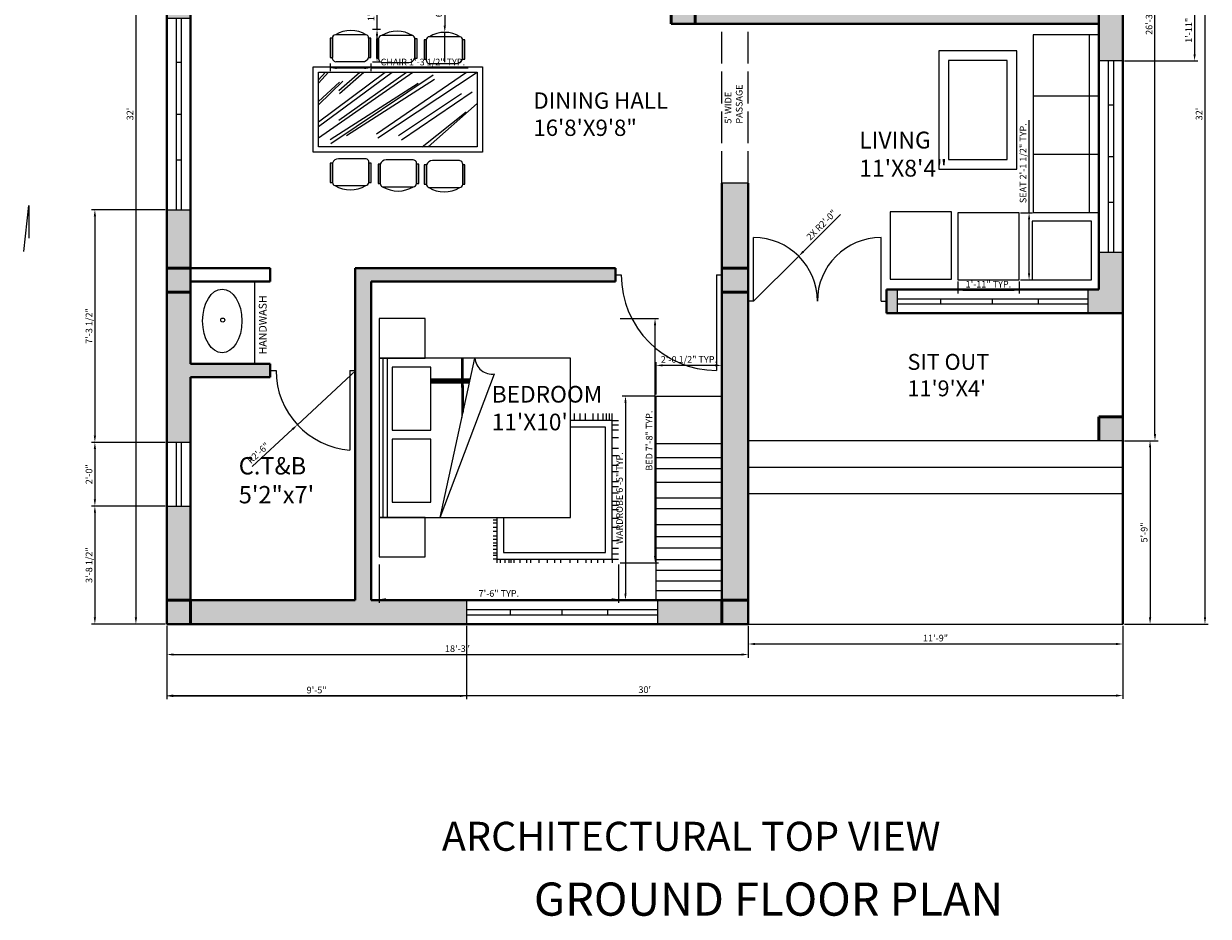
# Model space of a CAD drawing. Units: inches. Extents: x 599 to 1046, y 473 to 1020.
# Tile 1 of 2: x 599 to 1046, y 473 to 809. Entities that reach past the tile are written whole.
import ezdxf

# ---------------------------------------------------------------- set-up
doc = ezdxf.new("R2010")
doc.units = ezdxf.units.IN
doc.linetypes.add('ACAD_ISO02W100', pattern=[15, 12, -3])
for name, color, linetype, lineweight in [('A-ANNO-DIMS', 2, 'Continuous', 18), ('A-ANNO-MARK', 1, 'Continuous', 18), ('A-ANNO-TITL', 7, 'Continuous', 35), ('A-AREA-IDEN', 7, 'Continuous', 25), ('A-COLS', 7, 'Continuous', 50), ('A-COLS-PATT', 1, 'Continuous', 13), ('A-DOOR', 3, 'Continuous', 25), ('A-FLOR', 7, 'Continuous', 25), ('A-FLOR-CASE', 8, 'Continuous', 20), ('A-FLOR-FIXT', 9, 'Continuous', 18), ('A-FLOR-OVHD', 7, 'ACAD_ISO02W100', 18), ('A-FLOR-STRS', 7, 'Continuous', 25), ('A-FURN', 8, 'Continuous', 18), ('A-GLAZ', 4, 'Continuous', 18), ('A-WALL', 7, 'Continuous', 40), ('A-WALL-PATT', 252, 'Continuous', 13)]:
    doc.layers.add(name, color=color, linetype=linetype, lineweight=lineweight)
doc.styles.get("Standard").update_dxf_attribs({"font": 'arial.ttf'})
doc.dimstyles.new('ISO-25', dxfattribs={"dimtxt": 2.5, "dimasz": 2.5, "dimexe": 1.25, "dimexo": 0.625, "dimtad": 1, "dimdec": 0, "dimlunit": 3, "dimtxsty": 'Standard', "dimcen": 2.5, "dimadec": 0, "dimazin": 0, "dimtfac": 1, "dimtdec": 0, "dimtmove": 0, "dimatfit": 3, "dimfxl": 1, "dimarcsym": 0})

# ---------------------------------------------------------------- blocks, each defined once
blk = doc.blocks.new('*D2')
at = {"layer": 'A-ANNO-DIMS', "color": 0, "lineweight": -2, "transparency": 16777216}
for p, q in [((653.31, 582.63), (653.31, 570.57)), ((872.31, 582.63), (872.31, 570.57)), ((655.81, 571.82), (869.81, 571.82))]:
    blk.add_line(p, q, dxfattribs=at)
at = {"layer": 'A-ANNO-DIMS', "color": 0, "transparency": 16777216}
for points in [[(655.81, 572.23), (655.81, 571.4), (653.31, 571.82)], [(869.81, 572.23), (869.81, 571.4), (872.31, 571.82)]]:
    blk.add_solid(points, dxfattribs=at)
at = {"layer": 'Defpoints', "color": 0, "transparency": 16777216}
for p in [(653.31, 583.26), (872.31, 583.26), (872.31, 571.82)]:
    blk.add_point(p, dxfattribs=at)
at = {"layer": 'A-ANNO-DIMS', "color": 0, "transparency": 16777216, "insert": (762.81, 573.72), "char_height": 2.5, "attachment_point": 5}
blk.add_mtext('18\'-3"', dxfattribs=at)
blk = doc.blocks.new('*D3')
at = {"layer": 'A-ANNO-DIMS', "color": 0, "lineweight": -2, "transparency": 16777216}
for p, q in [((872.31, 582.63), (872.31, 574.53)), ((1013.31, 582.63), (1013.31, 574.53)), ((874.81, 575.78), (1010.81, 575.78))]:
    blk.add_line(p, q, dxfattribs=at)
at = {"layer": 'A-ANNO-DIMS', "color": 0, "transparency": 16777216}
for points in [[(874.81, 576.19), (874.81, 575.36), (872.31, 575.78)], [(1010.81, 576.19), (1010.81, 575.36), (1013.31, 575.78)]]:
    blk.add_solid(points, dxfattribs=at)
at = {"layer": 'Defpoints', "color": 0, "transparency": 16777216}
for p in [(872.31, 583.26), (1013.31, 583.26), (1013.31, 575.78)]:
    blk.add_point(p, dxfattribs=at)
at = {"layer": 'A-ANNO-DIMS', "color": 0, "transparency": 16777216, "insert": (942.81, 577.68), "char_height": 2.5, "attachment_point": 5}
blk.add_mtext('11\'-9"', dxfattribs=at)
blk = doc.blocks.new('*D4')
at = {"layer": 'A-ANNO-DIMS', "color": 0, "lineweight": -2, "transparency": 16777216}
for p, q in [((653.31, 582.63), (653.31, 555.11)), ((1013.31, 582.63), (1013.31, 555.11)), ((655.81, 556.36), (1010.81, 556.36))]:
    blk.add_line(p, q, dxfattribs=at)
at = {"layer": 'A-ANNO-DIMS', "color": 0, "transparency": 16777216}
for points in [[(655.81, 556.78), (655.81, 555.95), (653.31, 556.36)], [(1010.81, 556.78), (1010.81, 555.95), (1013.31, 556.36)]]:
    blk.add_solid(points, dxfattribs=at)
at = {"layer": 'Defpoints', "color": 0, "transparency": 16777216}
for p in [(653.31, 583.26), (1013.31, 583.26), (1013.31, 556.36)]:
    blk.add_point(p, dxfattribs=at)
at = {"layer": 'A-ANNO-DIMS', "color": 0, "transparency": 16777216, "insert": (833.31, 558.27), "char_height": 2.5, "attachment_point": 5}
blk.add_mtext("30'", dxfattribs=at)
blk = doc.blocks.new('*D5')
at = {"layer": 'A-ANNO-DIMS', "color": 0, "lineweight": -2, "transparency": 16777216}
for p, q in [((1013.94, 652.26), (1024.84, 652.26)), ((1023.59, 649.76), (1023.59, 585.76)), ((1013.94, 583.26), (1024.84, 583.26))]:
    blk.add_line(p, q, dxfattribs=at)
at = {"layer": 'A-ANNO-DIMS', "color": 0, "transparency": 16777216}
for points in [[(1023.17, 649.76), (1024.01, 649.76), (1023.59, 652.26)], [(1023.17, 585.76), (1024.01, 585.76), (1023.59, 583.26)]]:
    blk.add_solid(points, dxfattribs=at)
at = {"layer": 'Defpoints', "color": 0, "transparency": 16777216}
for p in [(1013.31, 652.26), (1013.31, 583.26), (1023.59, 583.26)]:
    blk.add_point(p, dxfattribs=at)
at = {"layer": 'A-ANNO-DIMS', "color": 0, "transparency": 16777216, "insert": (1021.69, 617.76), "char_height": 2.5, "attachment_point": 5, "rotation": 90}
blk.add_mtext('5\'-9"', dxfattribs=at)
blk = doc.blocks.new('*D6')
at = {"layer": 'A-ANNO-DIMS', "color": 0, "lineweight": -2, "transparency": 16777216}
for p, q in [((1013.94, 967.26), (1026.69, 967.26)), ((1025.44, 654.76), (1025.44, 964.76)), ((1013.94, 652.26), (1026.69, 652.26))]:
    blk.add_line(p, q, dxfattribs=at)
at = {"layer": 'A-ANNO-DIMS', "color": 0, "transparency": 16777216}
for points in [[(1025.02, 964.76), (1025.86, 964.76), (1025.44, 967.26)], [(1025.02, 654.76), (1025.86, 654.76), (1025.44, 652.26)]]:
    blk.add_solid(points, dxfattribs=at)
at = {"layer": 'Defpoints', "color": 0, "transparency": 16777216}
for p in [(1013.31, 967.26), (1025.44, 967.26), (1013.31, 652.26)]:
    blk.add_point(p, dxfattribs=at)
at = {"layer": 'A-ANNO-DIMS', "color": 0, "transparency": 16777216, "insert": (1023.54, 809.76), "char_height": 2.5, "attachment_point": 5, "rotation": 90}
blk.add_mtext('26\'-3"', dxfattribs=at)
blk = doc.blocks.new('*D7')
at = {"layer": 'A-ANNO-DIMS', "color": 0, "lineweight": -2, "transparency": 16777216}
for p, q in [((1013.94, 967.26), (1045.52, 967.26)), ((1044.27, 964.76), (1044.27, 585.76)), ((1013.94, 583.26), (1045.52, 583.26))]:
    blk.add_line(p, q, dxfattribs=at)
at = {"layer": 'A-ANNO-DIMS', "color": 0, "transparency": 16777216}
for points in [[(1043.86, 964.76), (1044.69, 964.76), (1044.27, 967.26)], [(1043.86, 585.76), (1044.69, 585.76), (1044.27, 583.26)]]:
    blk.add_solid(points, dxfattribs=at)
at = {"layer": 'Defpoints', "color": 0, "transparency": 16777216}
for p in [(1013.31, 967.26), (1013.31, 583.26), (1044.27, 583.26)]:
    blk.add_point(p, dxfattribs=at)
at = {"layer": 'A-ANNO-DIMS', "color": 0, "transparency": 16777216, "insert": (1042.37, 775.26), "char_height": 2.5, "attachment_point": 5, "rotation": 90}
blk.add_mtext("32'", dxfattribs=at)
blk = doc.blocks.new('*D8')
at = {"layer": 'A-ANNO-DIMS', "color": 0, "lineweight": -2, "transparency": 16777216}
for p, q in [((652.69, 967.26), (640.46, 967.26)), ((641.71, 964.76), (641.71, 585.76)), ((652.69, 583.26), (640.46, 583.26))]:
    blk.add_line(p, q, dxfattribs=at)
at = {"layer": 'A-ANNO-DIMS', "color": 0, "transparency": 16777216}
for points in [[(641.29, 964.76), (642.13, 964.76), (641.71, 967.26)], [(641.29, 585.76), (642.13, 585.76), (641.71, 583.26)]]:
    blk.add_solid(points, dxfattribs=at)
at = {"layer": 'Defpoints', "color": 0, "transparency": 16777216}
for p in [(653.31, 967.26), (641.71, 583.26), (653.31, 583.26)]:
    blk.add_point(p, dxfattribs=at)
at = {"layer": 'A-ANNO-DIMS', "color": 0, "transparency": 16777216, "insert": (639.81, 775.26), "char_height": 2.5, "attachment_point": 5, "rotation": 90}
blk.add_mtext("32'", dxfattribs=at)
blk = doc.blocks.new('CHAIR-DINING')
for points in [[(13.62, 10.12), (1.99, 10.12)], [(14.51, 1.64), (14.51, 8.94)], [(0.84, 8.92), (0.84, 1.64)], [(2.45, 0.02), (12.23, 0.02)]]:
    blk.add_lwpolyline(points)
for points in [[(0, 1.64), (0.84, 1.64), (0.84, 8.92), (0, 8.92)], [(14.51, 1.64), (15.34, 1.64), (15.34, 8.92), (14.51, 8.92)]]:
    blk.add_lwpolyline(points, close=True)
for centre, radius, start, end in [((2.04, 8.92), 1.2, 92.5102, 180), ((7.8, 0.53), 11.21, 58.7769, 121.2231), ((13.26, 8.93), 1.24, 359.5, 73.4744), ((2.2, 1.39), 1.39, 169.3227, 280.3594), ((12.23, 2.42), 2.4, 270, 341.0329)]:
    blk.add_arc(centre, radius, start, end)
blk = doc.blocks.new('BED-DOUBLE-ENSEMBLE')
for p, q in [((0, 77.06), (0, 17.06)), ((72, 77.06), (0, 77.06)), ((1.3, 77.06), (1.3, 17.06)), ((2.94, 77.06), (2.94, 17.06)), ((22.99, 17.06), (36, 77.06)), ((30.98, 77.06), (31.13, 54.62)), ((31.25, 55.16), (31.25, 77.06)), ((31.34, 55.57), (31.34, 77.06)), ((31.5, 77.06), (31.57, 56.64)), ((72, 17.06), (72, 77.06)), ((19.36, 69.18), (34.29, 69.19)), ((19.36, 68.78), (34.21, 68.79)), ((19.36, 68.38), (34.12, 68.39)), ((19.36, 68.04), (34.05, 68.05)), ((19.36, 67.69), (33.97, 67.7)), ((22.99, 17.06), (43.43, 71.06)), ((87.67, 53.54), (72, 53.54)), ((73.56, 53.54), (73.56, 56.2)), ((75.7, 53.54), (75.7, 56.2)), ((77.64, 53.54), (77.64, 56.2)), ((80.52, 53.54), (80.52, 56.2)), ((82.37, 53.54), (82.37, 56.2)), ((84.31, 53.54), (84.31, 56.2)), ((85.54, 53.54), (85.54, 56.2)), ((86.7, 53.54), (86.7, 56.2)), ((87.67, 53.54), (87.67, 56.2)), ((87.67, 1.32), (87.67, 53.54)), ((87.67, 53.54), (90.06, 53.54)), ((85.18, 51.05), (72, 51.05)), ((85.18, 3.81), (85.18, 51.05)), ((87.67, 51.93), (90.06, 51.93)), ((87.67, 50.03), (90.06, 50.03)), ((87.67, 47.15), (90.06, 47.15)), ((87.67, 43.16), (90.06, 43.16)), ((87.67, 40.35), (90.06, 40.35)), ((87.67, 36.69), (90.06, 36.69)), ((87.67, 34.33), (90.06, 34.33)), ((87.67, 30.54), (90.06, 30.54)), ((87.67, 28.71), (90.06, 28.71)), ((87.67, 26.29), (90.06, 26.29)), ((87.67, 23.15), (90.06, 23.15)), ((87.67, 21.64), (90.06, 21.64)), ((87.67, 20.07), (90.06, 20.07)), ((0, 17.06), (72, 17.06)), ((44.26, 16), (42.95, 16)), ((44.26, 14.88), (42.95, 14.88)), ((44.26, 17.06), (44.26, 1.32)), ((46.75, 17.06), (46.75, 3.81)), ((87.67, 16.74), (90.06, 16.74)), ((87.67, 13.4), (90.06, 13.4)), ((44.26, 13.3), (42.95, 13.3)), ((44.26, 11.8), (42.95, 11.8)), ((44.26, 10.06), (42.95, 10.06)), ((44.26, 8.76), (42.95, 8.76)), ((44.26, 7.43), (42.95, 7.43)), ((44.26, 6.36), (42.95, 6.36)), ((44.26, 4.95), (42.95, 4.95)), ((87.67, 8.34), (90.06, 8.34)), ((87.67, 5.52), (90.06, 5.52)), ((44.26, 3.6), (42.95, 3.6)), ((44.26, 2.68), (42.95, 2.68)), ((44.26, 1.32), (42.95, 1.32)), ((44.26, 1.32), (87.67, 1.32)), ((44.26, 1.32), (44.26, 0)), ((45.56, 1.32), (45.56, 0)), ((46.75, 3.81), (85.18, 3.81)), ((47.24, 1.32), (47.24, 0)), ((48.78, 1.32), (48.78, 0)), ((49.52, 1.32), (49.52, 0)), ((50.72, 1.32), (50.72, 0)), ((52.92, 1.32), (52.92, 0)), ((55.47, 1.32), (55.47, 0)), ((56.97, 1.32), (56.97, 0)), ((60.04, 1.32), (60.04, 0)), ((63.18, 1.32), (63.18, 0)), ((65.96, 1.32), (65.96, 0)), ((68.28, 1.32), (68.28, 0)), ((71.81, 1.32), (71.81, 0)), ((74.68, 1.32), (74.68, 0)), ((77.82, 1.32), (77.82, 0)), ((79.85, 1.32), (79.85, 0)), ((82.2, 1.32), (82.2, 0)), ((84.49, 1.32), (84.49, 0)), ((87.67, 3.36), (90.06, 3.36)), ((87.67, 1.32), (87.67, 0)), ((87.67, 1.32), (87.67, 0)), ((87.67, 1.32), (90.06, 1.32))]:
    blk.add_line(p, q)
for points in [[(0, 77.06), (17.35, 77.06), (17.35, 91.9), (0, 91.9)], [(4.8, 49.9), (19.36, 49.9), (19.36, 73.67), (4.8, 73.67)], [(4.8, 22.77), (19.36, 22.77), (19.36, 46.55), (4.8, 46.55)], [(0, 2.22), (17.35, 2.22), (17.35, 17.06), (0, 17.06)]]:
    blk.add_lwpolyline(points, close=True)
blk.add_arc((42.53, 77.54), 6.55, 184.2463, 277.8518)
blk = doc.blocks.new('WARDROBE-BEDROOM')
for p, q in [((0, 73.38), (24.73, 73.38)), ((0, 69.72), (24.73, 69.72)), ((0, 65.72), (24.73, 65.72)), ((0, 61.6), (24.73, 61.6)), ((0, 57.26), (24.73, 57.26)), ((0, 52.97), (24.73, 52.97)), ((0, 48.49), (24.73, 48.49)), ((0, 42.41), (24.73, 42.41)), ((0, 38.43), (24.73, 38.43)), ((0, 32.59), (24.73, 32.59)), ((0, 27.44), (24.73, 27.44)), ((0, 23.23), (24.73, 23.23)), ((0, 18.05), (24.73, 18.05))]:
    blk.add_line(p, q)
blk.add_lwpolyline([(0, 76.86), (24.73, 76.86), (24.73, 0), (0, 0)], close=True)
blk = doc.blocks.new('WIN-72IN')
for p, q in [((3.5, 72), (3.5, 0)), ((5.5, 72), (5.5, 0)), ((3.5, 55.48), (5.5, 55.48)), ((3.5, 36), (5.5, 36)), ((3.5, 18.8), (5.5, 18.8))]:
    blk.add_line(p, q)
blk.add_lwpolyline([(0, 72), (0, 0), (9, 0), (9, 72)], close=True)
blk = doc.blocks.new('DOOR-SINGLE-36IN')
for p, q in [((0, 36), (2.13, 36)), ((38, 36), (38, 0)), ((38, 36), (40, 36))]:
    blk.add_line(p, q)
blk.add_arc((38.13, 36), 36, 180, 269.8005)
blk = doc.blocks.new('SEAT-LOUNGE')
blk.add_lwpolyline([(0, 0), (23.03, 0), (23.03, 25.27), (0, 25.27)], close=True)
blk = doc.blocks.new('*D17')
at = {"layer": 'A-ANNO-DIMS', "color": 0, "lineweight": -2, "transparency": 16777216}
for p, q in [((714.85, 794.26), (714.85, 791.34)), ((730.19, 794.26), (730.19, 791.34)), ((717.35, 792.59), (727.69, 792.59)), ((730.19, 792.59), (766.82, 792.59))]:
    blk.add_line(p, q, dxfattribs=at)
at = {"layer": 'A-ANNO-DIMS', "color": 0, "transparency": 16777216}
for points in [[(717.35, 793), (717.35, 792.17), (714.85, 792.59)], [(727.69, 793), (727.69, 792.17), (730.19, 792.59)]]:
    blk.add_solid(points, dxfattribs=at)
at = {"layer": 'Defpoints', "color": 0, "transparency": 16777216}
for p in [(714.85, 794.89), (730.19, 794.89), (730.19, 792.59)]:
    blk.add_point(p, dxfattribs=at)
at = {"layer": 'A-ANNO-DIMS', "color": 0, "transparency": 16777216, "insert": (749.76, 794.5), "char_height": 2.5, "attachment_point": 5}
blk.add_mtext('CHAIR 1\'-3 1/2" TYP.', dxfattribs=at)
blk = doc.blocks.new('*D18')
at = {"layer": 'A-ANNO-DIMS', "color": 0, "lineweight": -2, "transparency": 16777216}
for p, q in [((732.5, 807.24), (732.5, 831.82)), ((730.82, 807.24), (733.75, 807.24)), ((732.5, 797.39), (732.5, 804.74)), ((730.82, 794.89), (733.75, 794.89))]:
    blk.add_line(p, q, dxfattribs=at)
at = {"layer": 'A-ANNO-DIMS', "color": 0, "transparency": 16777216}
for points in [[(732.08, 804.74), (732.91, 804.74), (732.5, 807.24)], [(732.08, 797.39), (732.91, 797.39), (732.5, 794.89)]]:
    blk.add_solid(points, dxfattribs=at)
at = {"layer": 'Defpoints', "color": 0, "transparency": 16777216}
for p in [(730.19, 807.24), (732.5, 807.24), (730.19, 794.89)]:
    blk.add_point(p, dxfattribs=at)
at = {"layer": 'A-ANNO-DIMS', "color": 0, "transparency": 16777216, "insert": (730.58, 820.78), "char_height": 2.5, "attachment_point": 5, "rotation": 90}
blk.add_mtext('1\'-0 1/2" TYP.', dxfattribs=at)
blk = doc.blocks.new('*D23')
at = {"layer": 'A-ANNO-DIMS', "color": 0, "lineweight": -2, "transparency": 16777216}
for p, q in [((824.03, 698.27), (838.44, 698.27)), ((837.19, 608.87), (837.19, 695.77)), ((824.03, 606.37), (838.44, 606.37))]:
    blk.add_line(p, q, dxfattribs=at)
at = {"layer": 'A-ANNO-DIMS', "color": 0, "transparency": 16777216}
for points in [[(836.77, 695.77), (837.6, 695.77), (837.19, 698.27)], [(836.77, 608.87), (837.6, 608.87), (837.19, 606.37)]]:
    blk.add_solid(points, dxfattribs=at)
at = {"layer": 'Defpoints', "color": 0, "transparency": 16777216}
for p in [(823.4, 698.27), (837.19, 698.27), (823.4, 606.37)]:
    blk.add_point(p, dxfattribs=at)
at = {"layer": 'A-ANNO-DIMS', "color": 0, "transparency": 16777216, "insert": (835.29, 652.32), "char_height": 2.5, "attachment_point": 5, "rotation": 90}
blk.add_mtext('BED 7\'-8" TYP.', dxfattribs=at)
blk = doc.blocks.new('*D24')
at = {"layer": 'A-ANNO-DIMS', "color": 0, "lineweight": -2, "transparency": 16777216}
for p, q in [((733.34, 605.74), (733.34, 591.33)), ((823.4, 605.74), (823.4, 591.33)), ((735.84, 592.58), (820.9, 592.58))]:
    blk.add_line(p, q, dxfattribs=at)
at = {"layer": 'A-ANNO-DIMS', "color": 0, "transparency": 16777216}
for points in [[(735.84, 593), (735.84, 592.16), (733.34, 592.58)], [(820.9, 593), (820.9, 592.16), (823.4, 592.58)]]:
    blk.add_solid(points, dxfattribs=at)
at = {"layer": 'Defpoints', "color": 0, "transparency": 16777216}
for p in [(733.34, 606.37), (823.4, 606.37), (823.4, 592.58)]:
    blk.add_point(p, dxfattribs=at)
at = {"layer": 'A-ANNO-DIMS', "color": 0, "transparency": 16777216, "insert": (778.37, 594.48), "char_height": 2.5, "attachment_point": 5}
blk.add_mtext('7\'-6" TYP.', dxfattribs=at)
blk = doc.blocks.new('*D25')
at = {"layer": 'A-ANNO-DIMS', "color": 0, "lineweight": -2, "transparency": 16777216}
for p, q in [((836.96, 669.12), (824.81, 669.12)), ((826.06, 666.62), (826.06, 594.76)), ((836.96, 592.26), (824.81, 592.26))]:
    blk.add_line(p, q, dxfattribs=at)
at = {"layer": 'A-ANNO-DIMS', "color": 0, "transparency": 16777216}
for points in [[(825.64, 666.62), (826.47, 666.62), (826.06, 669.12)], [(825.64, 594.76), (826.47, 594.76), (826.06, 592.26)]]:
    blk.add_solid(points, dxfattribs=at)
at = {"layer": 'Defpoints', "color": 0, "transparency": 16777216}
for p in [(837.59, 669.12), (826.06, 592.26), (837.59, 592.26)]:
    blk.add_point(p, dxfattribs=at)
at = {"layer": 'A-ANNO-DIMS', "color": 0, "transparency": 16777216, "insert": (824.14, 630.69), "char_height": 2.5, "attachment_point": 5, "rotation": 90}
blk.add_mtext('WARDROBE 6\'-5" TYP.', dxfattribs=at)
blk = doc.blocks.new('*D26')
at = {"layer": 'A-ANNO-DIMS', "color": 0, "lineweight": -2, "transparency": 16777216}
for p, q in [((837.59, 669.74), (837.59, 681.9)), ((859.81, 680.65), (840.09, 680.65)), ((862.31, 669.74), (862.31, 681.9))]:
    blk.add_line(p, q, dxfattribs=at)
at = {"layer": 'A-ANNO-DIMS', "color": 0, "transparency": 16777216}
for points in [[(840.09, 681.06), (840.09, 680.23), (837.59, 680.65)], [(859.81, 681.06), (859.81, 680.23), (862.31, 680.65)]]:
    blk.add_solid(points, dxfattribs=at)
at = {"layer": 'Defpoints', "color": 0, "transparency": 16777216}
for p in [(837.59, 680.65), (837.59, 669.12), (862.31, 669.12)]:
    blk.add_point(p, dxfattribs=at)
at = {"layer": 'A-ANNO-DIMS', "color": 0, "transparency": 16777216, "insert": (849.95, 682.57), "char_height": 2.5, "attachment_point": 5}
blk.add_mtext('2\'-0 1/2" TYP.', dxfattribs=at)
blk = doc.blocks.new('*D29')
at = {"layer": 'A-ANNO-DIMS', "color": 0, "lineweight": -2, "transparency": 16777216}
for p, q in [((978.03, 738.07), (978.03, 772.96)), ((974.86, 738.07), (979.28, 738.07)), ((978.03, 715.3), (978.03, 735.57)), ((974.86, 712.8), (979.28, 712.8))]:
    blk.add_line(p, q, dxfattribs=at)
at = {"layer": 'A-ANNO-DIMS', "color": 0, "transparency": 16777216}
for points in [[(977.61, 735.57), (978.45, 735.57), (978.03, 738.07)], [(977.61, 715.3), (978.45, 715.3), (978.03, 712.8)]]:
    blk.add_solid(points, dxfattribs=at)
at = {"layer": 'Defpoints', "color": 0, "transparency": 16777216}
for p in [(974.24, 738.07), (978.03, 738.07), (974.24, 712.8)]:
    blk.add_point(p, dxfattribs=at)
at = {"layer": 'A-ANNO-DIMS', "color": 0, "transparency": 16777216, "insert": (976.11, 756.76), "char_height": 2.5, "attachment_point": 5, "rotation": 90}
blk.add_mtext('SEAT 2\'-1 1/2" TYP.', dxfattribs=at)
blk = doc.blocks.new('*D30')
at = {"layer": 'A-ANNO-DIMS', "color": 0, "lineweight": -2, "transparency": 16777216}
for p, q in [((951.21, 712.17), (951.21, 707.76)), ((974.24, 712.17), (974.24, 707.76)), ((953.71, 709.01), (971.74, 709.01))]:
    blk.add_line(p, q, dxfattribs=at)
at = {"layer": 'A-ANNO-DIMS', "color": 0, "transparency": 16777216}
for points in [[(953.71, 709.42), (953.71, 708.59), (951.21, 709.01)], [(971.74, 709.42), (971.74, 708.59), (974.24, 709.01)]]:
    blk.add_solid(points, dxfattribs=at)
at = {"layer": 'Defpoints', "color": 0, "transparency": 16777216}
for p in [(951.21, 712.8), (974.24, 712.8), (974.24, 709.01)]:
    blk.add_point(p, dxfattribs=at)
at = {"layer": 'A-ANNO-DIMS', "color": 0, "transparency": 16777216, "insert": (962.72, 710.89), "char_height": 2.5, "attachment_point": 5}
blk.add_mtext('1\'-11" TYP.', dxfattribs=at)
blk = doc.blocks.new('*D35')
at = {"layer": 'A-ANNO-DIMS', "color": 0, "lineweight": -2, "transparency": 16777216}
for p, q in [((652.69, 651.68), (625.01, 651.68)), ((626.26, 649.18), (626.26, 630.18)), ((652.69, 627.68), (625.01, 627.68))]:
    blk.add_line(p, q, dxfattribs=at)
at = {"layer": 'A-ANNO-DIMS', "color": 0, "transparency": 16777216}
for points in [[(625.85, 649.18), (626.68, 649.18), (626.26, 651.68)], [(625.85, 630.18), (626.68, 630.18), (626.26, 627.68)]]:
    blk.add_solid(points, dxfattribs=at)
at = {"layer": 'Defpoints', "color": 0, "transparency": 16777216}
for p in [(653.31, 651.68), (626.26, 627.68), (653.31, 627.68)]:
    blk.add_point(p, dxfattribs=at)
at = {"layer": 'A-ANNO-DIMS', "color": 0, "transparency": 16777216, "insert": (624.36, 639.68), "char_height": 2.5, "attachment_point": 5, "rotation": 90}
blk.add_mtext('2\'-0"', dxfattribs=at)
blk = doc.blocks.new('*D36')
at = {"layer": 'A-ANNO-DIMS', "color": 0, "lineweight": -2, "transparency": 16777216}
for p, q in [((652.69, 627.68), (625.01, 627.68)), ((626.26, 625.18), (626.26, 585.76)), ((652.69, 583.26), (625.01, 583.26))]:
    blk.add_line(p, q, dxfattribs=at)
at = {"layer": 'A-ANNO-DIMS', "color": 0, "transparency": 16777216}
for points in [[(625.85, 625.18), (626.68, 625.18), (626.26, 627.68)], [(625.85, 585.76), (626.68, 585.76), (626.26, 583.26)]]:
    blk.add_solid(points, dxfattribs=at)
at = {"layer": 'Defpoints', "color": 0, "transparency": 16777216}
for p in [(653.31, 627.68), (626.26, 583.26), (653.31, 583.26)]:
    blk.add_point(p, dxfattribs=at)
at = {"layer": 'A-ANNO-DIMS', "color": 0, "transparency": 16777216, "insert": (624.35, 605.47), "char_height": 2.5, "attachment_point": 5, "rotation": 90}
blk.add_mtext('3\'-8 1/2"', dxfattribs=at)
blk = doc.blocks.new('*D37')
at = {"layer": 'A-ANNO-DIMS', "color": 0, "lineweight": -2, "transparency": 16777216}
for p, q in [((652.69, 739.26), (625.01, 739.26)), ((626.26, 736.76), (626.26, 654.18)), ((652.69, 651.68), (625.01, 651.68))]:
    blk.add_line(p, q, dxfattribs=at)
at = {"layer": 'A-ANNO-DIMS', "color": 0, "transparency": 16777216}
for points in [[(625.85, 736.76), (626.68, 736.76), (626.26, 739.26)], [(625.85, 654.18), (626.68, 654.18), (626.26, 651.68)]]:
    blk.add_solid(points, dxfattribs=at)
at = {"layer": 'Defpoints', "color": 0, "transparency": 16777216}
for p in [(653.31, 739.26), (626.26, 651.68), (653.31, 651.68)]:
    blk.add_point(p, dxfattribs=at)
at = {"layer": 'A-ANNO-DIMS', "color": 0, "transparency": 16777216, "insert": (624.35, 695.47), "char_height": 2.5, "attachment_point": 5, "rotation": 90}
blk.add_mtext('7\'-3 1/2"', dxfattribs=at)
blk = doc.blocks.new('*D39')
at = {"layer": 'A-ANNO-DIMS', "color": 0, "lineweight": -2, "transparency": 16777216}
for p, q in [((653.31, 582.63), (653.31, 554.96)), ((766.2, 582.63), (766.2, 554.96)), ((655.81, 556.21), (763.7, 556.21))]:
    blk.add_line(p, q, dxfattribs=at)
at = {"layer": 'A-ANNO-DIMS', "color": 0, "transparency": 16777216}
for points in [[(655.81, 556.63), (655.81, 555.79), (653.31, 556.21)], [(763.7, 556.63), (763.7, 555.79), (766.2, 556.21)]]:
    blk.add_solid(points, dxfattribs=at)
at = {"layer": 'Defpoints', "color": 0, "transparency": 16777216}
for p in [(653.31, 583.26), (766.2, 583.26), (766.2, 556.21)]:
    blk.add_point(p, dxfattribs=at)
at = {"layer": 'A-ANNO-DIMS', "color": 0, "transparency": 16777216, "insert": (709.76, 558.11), "char_height": 2.5, "attachment_point": 5}
blk.add_mtext('9\'-5"', dxfattribs=at)
blk = doc.blocks.new('*D42')
at = {"layer": 'A-ANNO-DIMS', "color": 0, "lineweight": -2, "transparency": 16777216}
for p, q in [((1013.94, 818.26), (1041.61, 818.26)), ((1040.36, 815.76), (1040.36, 797.76)), ((1013.94, 795.26), (1041.61, 795.26))]:
    blk.add_line(p, q, dxfattribs=at)
at = {"layer": 'A-ANNO-DIMS', "color": 0, "transparency": 16777216}
for points in [[(1039.95, 815.76), (1040.78, 815.76), (1040.36, 818.26)], [(1039.95, 797.76), (1040.78, 797.76), (1040.36, 795.26)]]:
    blk.add_solid(points, dxfattribs=at)
at = {"layer": 'Defpoints', "color": 0, "transparency": 16777216}
for p in [(1013.31, 818.26), (1013.31, 795.26), (1040.36, 795.26)]:
    blk.add_point(p, dxfattribs=at)
at = {"layer": 'A-ANNO-DIMS', "color": 0, "transparency": 16777216, "insert": (1038.48, 806.76), "char_height": 2.5, "attachment_point": 5, "rotation": 90}
blk.add_mtext('1\'-11"', dxfattribs=at)
blk = doc.blocks.new('*D43')
at = {"layer": 'A-ANNO-DIMS', "color": 0, "lineweight": -2, "transparency": 16777216}
for p, q in [((724.57, 678.76), (702.52, 658.3)), ((685.51, 642.53), (700.68, 656.6))]:
    blk.add_line(p, q, dxfattribs=at)
at = {"layer": 'A-ANNO-DIMS', "color": 0, "transparency": 16777216}
blk.add_solid([(700.4, 656.91), (700.97, 656.29), (702.52, 658.3)], dxfattribs=at)
at = {"layer": 'Defpoints', "color": 0, "transparency": 16777216}
for p in [(724.57, 678.76), (702.52, 658.3)]:
    blk.add_point(p, dxfattribs=at)
at = {"layer": 'A-ANNO-DIMS', "color": 0, "transparency": 16777216, "insert": (687.99, 647.42), "char_height": 2.5, "attachment_point": 5, "rotation": 42.8473}
blk.add_mtext('R2\'-6"', dxfattribs=at)
blk = doc.blocks.new('*D45')
at = {"layer": 'A-ANNO-DIMS', "color": 0, "lineweight": -2, "transparency": 16777216}
for p, q in [((907.02, 737.49), (893.05, 723.53)), ((874.31, 704.79), (891.29, 721.76))]:
    blk.add_line(p, q, dxfattribs=at)
at = {"layer": 'A-ANNO-DIMS', "color": 0, "transparency": 16777216}
blk.add_solid([(892.76, 723.82), (893.35, 723.23), (891.29, 721.76)], dxfattribs=at)
at = {"layer": 'Defpoints', "color": 0, "transparency": 16777216}
for p in [(891.29, 721.76), (874.31, 704.79)]:
    blk.add_point(p, dxfattribs=at)
at = {"layer": 'A-ANNO-DIMS', "color": 0, "transparency": 16777216, "insert": (900.12, 733.29), "char_height": 2.5, "attachment_point": 5, "rotation": 44.9991}
blk.add_mtext('2X R2\'-0"', dxfattribs=at)
blk = doc.blocks.new('*D47')
at = {"layer": 'A-ANNO-DIMS', "color": 0, "lineweight": -2, "transparency": 16777216}
for p, q in [((758.01, 828.61), (758.01, 808.5)), ((758.01, 794.78), (758.01, 806))]:
    blk.add_line(p, q, dxfattribs=at)
at = {"layer": 'A-ANNO-DIMS', "color": 0, "transparency": 16777216}
blk.add_solid([(757.59, 808.5), (758.43, 808.5), (758.01, 806)], dxfattribs=at)
at = {"layer": 'Defpoints', "color": 0, "transparency": 16777216}
for p in [(758.01, 806), (758.01, 794.78)]:
    blk.add_point(p, dxfattribs=at)
at = {"layer": 'A-ANNO-DIMS', "color": 0, "transparency": 16777216, "insert": (756.11, 819.81), "char_height": 2.5, "attachment_point": 5, "rotation": 89.9975}
blk.add_mtext('6X R0\'-11"', dxfattribs=at)

msp = doc.modelspace()

# ---------------------------------------------------------------- hatches: boundary and pattern name
at = {"layer": 'A-COLS-PATT'}
h = msp.add_hatch(color=256, dxfattribs=at)
h.dxf.hatch_style = 1
h.paths.add_polyline_path([(662.31, 967.26), (653.31, 967.26), (653.31, 958.26), (662.31, 958.26)])
h.paths.add_polyline_path([(852.31, 967.26), (843.31, 967.26), (843.31, 958.26), (852.31, 958.26)])
h.paths.add_polyline_path([(771.31, 842.26), (762.31, 842.26), (762.31, 833.26), (771.31, 833.26)])
h.paths.add_polyline_path([(771.31, 967.26), (762.31, 967.26), (762.31, 958.26), (771.31, 958.26)])
h.paths.add_polyline_path([(662.31, 842.26), (653.31, 842.26), (653.31, 833.26), (662.31, 833.26)])
h.paths.add_polyline_path([(852.31, 818.26), (843.31, 818.26), (843.31, 809.26), (852.31, 809.26)])
h.paths.add_polyline_path([(1013.31, 967.26), (1004.31, 967.26), (1004.31, 958.26), (1013.31, 958.26)])
h.paths.add_polyline_path([(662.31, 592.26), (653.31, 592.26), (653.31, 583.26), (662.31, 583.26)])
h = msp.add_hatch(color=256, dxfattribs=at)
h.dxf.hatch_style = 1
h.paths.add_polyline_path([(662.31, 717.26), (653.31, 717.26), (653.31, 708.26), (662.31, 708.26)])
h.paths.add_polyline_path([(872.31, 717.26), (862.31, 717.26), (862.31, 708.26), (872.31, 708.26)])
h.paths.add_polyline_path([(872.31, 592.26), (862.31, 592.26), (862.31, 583.26), (872.31, 583.26)])
h.paths.add_polyline_path([(1013.31, 661.26), (1004.31, 661.26), (1004.31, 652.26), (1013.31, 652.26)])
h.paths.add_polyline_path([(1013.31, 818.26), (1004.31, 818.26), (1004.31, 809.26), (1013.31, 809.26)])
at = {"layer": 'A-WALL-PATT'}
h = msp.add_hatch(color=256, dxfattribs=at)
h.dxf.hatch_style = 1
h.paths.add_polyline_path([(662.31, 865.76), (653.31, 865.76), (653.31, 842.26), (662.31, 842.26)])
h.paths.add_polyline_path([(662.31, 833.26), (653.31, 833.26), (653.31, 811.26), (662.31, 811.26)])
h.paths.add_polyline_path([(722.31, 838.26), (662.31, 838.26), (662.31, 833.26), (722.31, 833.26)])
h.paths.add_polyline_path([(662.31, 739.26), (653.31, 739.26), (653.31, 717.26), (662.31, 717.26)])
h.paths.add_polyline_path([(662.31, 708.26), (653.31, 708.26), (653.31, 651.68), (662.31, 651.68), (662.31, 676.26), (692.31, 676.26), (692.31, 681.26), (662.31, 681.26)])
h.paths.add_polyline_path([(662.31, 627.68), (653.31, 627.68), (653.31, 592.26), (662.31, 592.26)])
h.paths.add_polyline_path([(766.2, 592.26), (730.31, 592.26), (730.31, 712.26), (822.31, 712.26), (822.31, 717.26), (724.31, 717.26), (724.31, 676.26), (724.31, 592.26), (662.31, 592.26), (662.31, 583.26), (766.2, 583.26)])
h.paths.add_polyline_path([(872.31, 708.26), (862.31, 708.26), (862.31, 592.26), (872.31, 592.26)])
h.paths.add_polyline_path([(1013.31, 809.26), (1004.31, 809.26), (1004.31, 795.26), (1013.31, 795.26)])
h.paths.add_polyline_path([(1004.31, 814.26), (852.31, 814.26), (852.31, 809.26), (1004.31, 809.26)])
h.paths.add_polyline_path([(843.31, 967.26), (771.31, 967.26), (771.31, 958.26), (843.31, 958.26)])
h.paths.add_polyline_path([(771.31, 958.26), (766.31, 958.26), (766.31, 842.26), (771.31, 842.26)])
h.paths.add_polyline_path([(722.31, 967.26), (662.31, 967.26), (662.31, 958.26), (722.31, 958.26)])
h.paths.add_polyline_path([(662.31, 958.26), (653.31, 958.26), (653.31, 925.76), (662.31, 925.76)])
h.paths.add_polyline_path([(896.33, 967.26), (852.31, 967.26), (852.31, 958.26), (873.04, 958.26), (896.33, 958.26)])
h.paths.add_polyline_path([(1004.31, 967.26), (968.33, 967.26), (968.33, 958.26), (1004.31, 958.26)])
h.paths.add_polyline_path([(1013.31, 917.26), (1004.31, 917.26), (1004.31, 859.26), (1013.31, 859.26)])
h.paths.add_polyline_path([(1013.31, 723.26), (1004.31, 723.26), (1004.31, 709.26), (1000.32, 709.26), (1000.32, 700.26), (1013.31, 700.26)])
h.paths.add_polyline_path([(872.31, 749.26), (862.31, 749.26), (862.31, 717.26), (872.31, 717.26)])
h.paths.add_polyline_path([(862.31, 592.26), (838.2, 592.26), (838.2, 583.26), (862.31, 583.26)])
h.paths.add_polyline_path([(928.32, 709.26), (924.31, 709.26), (924.31, 700.26), (928.32, 700.26)])

# ---------------------------------------------------------------- linework, layer by layer
at = {"layer": 'A-ANNO-MARK'}
for p, q in [((599.45, 723.54), (601.34, 740.77)), ((601.34, 740.77), (601.34, 728.54))]:
    msp.add_line(p, q, dxfattribs=at)
at = {"layer": 'A-COLS'}
for p, q in [((843.31, 809.26), (843.31, 818.26)), ((852.31, 809.26), (852.31, 818.26)), ((662.31, 717.26), (653.31, 717.26)), ((872.31, 717.26), (862.31, 717.26)), ((653.31, 708.26), (662.31, 708.26)), ((862.31, 708.26), (872.31, 708.26)), ((1013.31, 661.26), (1004.31, 661.26)), ((1004.31, 661.26), (1004.31, 652.26)), ((662.31, 592.26), (653.31, 592.26)), ((662.31, 583.26), (662.31, 592.26)), ((872.31, 592.26), (862.31, 592.26)), ((862.31, 592.26), (862.31, 583.26))]:
    msp.add_line(p, q, dxfattribs=at)
at = {"layer": 'A-DOOR'}
for p, q in [((874.31, 704.79), (874.31, 728.79)), ((922.31, 704.79), (922.31, 728.79)), ((874.31, 704.79), (872.31, 704.79)), ((922.31, 704.79), (924.31, 704.79)), ((692.31, 678.76), (694.49, 678.76)), ((722.31, 678.76), (722.31, 648.76)), ((722.31, 678.76), (724.31, 678.76))]:
    msp.add_line(p, q, dxfattribs=at)
for centre, radius, start, end in [((874.31, 704.79), 24, 0, 90), ((922.31, 704.79), 24, 90, 180), ((724.57, 678.76), 30.08, 180, 265.6957)]:
    msp.add_arc(centre, radius, start, end, dxfattribs=at)
at = {"layer": 'A-FLOR'}
msp.add_line((872.31, 583.26), (1013.31, 583.26), dxfattribs=at)
at = {"layer": 'A-FLOR-CASE'}
msp.add_line((686.31, 712.26), (686.31, 681.26), dxfattribs=at)
at = {"layer": 'A-FLOR-FIXT'}
msp.add_circle((674.4, 697.72), 0.745, dxfattribs=at)
msp.add_ellipse((674.23, 697.38), major_axis=(0, 11.99), ratio=0.61768, dxfattribs=at)
at = {"layer": 'A-FLOR-OVHD'}
for p, q in [((862.31, 749.26), (862.31, 809.26)), ((872.31, 749.26), (872.31, 809.26)), ((872.31, 749.26), (862.31, 749.26))]:
    msp.add_line(p, q, dxfattribs=at)
at = {"layer": 'A-FLOR-STRS'}
for p, q in [((1013.31, 652.26), (872.31, 652.26)), ((1013.31, 642.26), (872.31, 642.26)), ((1013.31, 632.26), (872.31, 632.26))]:
    msp.add_line(p, q, dxfattribs=at)
at = {"layer": 'A-FURN'}
for p, q in [((1000.83, 738.24), (1000.83, 805.04)), ((710.43, 788.09), (713.1, 791.06)), ((710.43, 786.86), (714.19, 791.06)), ((710.43, 770.62), (738.26, 791.06)), ((710.43, 772.35), (735.54, 791.06)), ((710.43, 766.32), (746.02, 791.06)), ((715.06, 764.18), (753.7, 790.01)), ((718.07, 784.15), (726.04, 791.06)), ((718.11, 772.93), (743.63, 791.06)), ((718.36, 783.04), (727.48, 791.06)), ((732.27, 767.82), (766.14, 791.06)), ((732.81, 766.24), (770.24, 791.06)), ((710.43, 778.74), (719.68, 787.57)), ((710.43, 779.92), (718.36, 787.28)), ((714.87, 765.7), (747.98, 786.85)), ((721.05, 767.18), (754.15, 788.33)), ((740.57, 767.24), (764.32, 782.98)), ((741.71, 765.53), (768.3, 783.66)), ((979.54, 782.16), (1004.31, 782.16)), ((751.8, 762.85), (770.24, 779.2)), ((749.49, 762.85), (766.09, 776.14)), ((979.54, 760.14), (1004.31, 760.14))]:
    msp.add_line(p, q, dxfattribs=at)
for points in [[(979.54, 738.24), (1004.31, 738.24), (1004.31, 805.04), (979.54, 805.04)], [(944.11, 754.51), (973.37, 754.51), (973.37, 798.99), (944.11, 798.99)], [(947.74, 758.14), (969.74, 758.14), (969.74, 795.35), (947.74, 795.35)], [(708.43, 793.06), (772.24, 793.06), (772.24, 760.85), (708.43, 760.85)], [(710.43, 791.06), (770.24, 791.06), (770.24, 762.85), (710.43, 762.85)], [(979.15, 712.82), (1001.6, 712.82), (1001.6, 734.91), (979.15, 734.91)]]:
    msp.add_lwpolyline(points, close=True, dxfattribs=at)
at = {"layer": 'A-GLAZ'}
for p, q in [((656.81, 651.68), (656.81, 627.68)), ((658.81, 651.68), (658.81, 627.68))]:
    msp.add_line(p, q, dxfattribs=at)
msp.add_lwpolyline([(653.31, 651.68), (653.31, 627.68), (662.31, 627.68), (662.31, 651.68)], close=True, dxfattribs=at)
at = {"layer": 'A-WALL'}
for p, q in [((653.31, 967.26), (653.31, 583.26)), ((1013.31, 583.26), (1013.31, 967.26)), ((1004.31, 809.26), (1004.31, 958.26)), ((662.31, 833.26), (662.31, 717.26)), ((1004.31, 809.26), (843.31, 809.26)), ((1004.31, 709.26), (1004.31, 809.26)), ((862.31, 592.26), (862.31, 749.26)), ((872.31, 583.26), (872.31, 749.26)), ((662.31, 717.26), (692.31, 717.26)), ((662.31, 717.26), (662.31, 681.26)), ((692.31, 712.26), (692.31, 717.26)), ((724.31, 717.26), (724.31, 676.26)), ((724.31, 717.26), (822.31, 717.26)), ((822.31, 712.26), (822.31, 717.26)), ((662.31, 712.26), (692.31, 712.26)), ((730.31, 712.26), (730.31, 592.26)), ((730.31, 712.26), (822.31, 712.26)), ((1004.31, 709.26), (924.31, 709.26)), ((924.31, 700.26), (924.31, 709.26)), ((1013.31, 700.26), (924.31, 700.26)), ((662.31, 681.26), (692.31, 681.26)), ((692.31, 676.26), (692.31, 681.26)), ((662.31, 676.26), (692.31, 676.26)), ((662.31, 676.26), (662.31, 592.26)), ((724.31, 676.26), (724.31, 592.26)), ((662.31, 592.26), (724.31, 592.26)), ((730.31, 592.26), (862.31, 592.26)), ((653.31, 583.26), (872.31, 583.26))]:
    msp.add_line(p, q, dxfattribs=at)

# ---------------------------------------------------------------- block references
at = {"layer": 'A-DOOR'}
msp.add_blockref('DOOR-SINGLE-36IN', (822.31, 678.76), dxfattribs=at)
at = {"layer": 'A-FLOR-CASE', "rotation": 180}
msp.add_blockref('WARDROBE-BEDROOM', (862.31, 669.12), dxfattribs=at)
at = {"layer": 'A-FURN'}
for name, p in [('CHAIR-DINING', (714.85, 794.95)), ('CHAIR-DINING', (732.25, 794.68)), ('CHAIR-DINING', (750.21, 794.25)), ('SEAT-LOUNGE', (925.75, 713.14)), ('SEAT-LOUNGE', (951.21, 712.8)), ('BED-DOUBLE-ENSEMBLE', (733.34, 606.36))]:
    msp.add_blockref(name, p, dxfattribs=at)
at = {"layer": 'A-FURN', "rotation": 180}
for p in [(730.25, 758.44), (748.21, 758.01), (765.61, 757.74)]:
    msp.add_blockref('CHAIR-DINING', p, dxfattribs=at)
at = {"layer": 'A-GLAZ'}
for p in [(653.31, 739.26), (1004.31, 723.26)]:
    msp.add_blockref('WIN-72IN', p, dxfattribs=at)
for p, rotation in [((1000.32, 700.26), 90.00000000000038), ((838.2, 583.26), 89.99999999999999)]:
    msp.add_blockref('WIN-72IN', p, dxfattribs=dict(at, rotation=rotation))

# ---------------------------------------------------------------- texts
at = {"layer": 'A-ANNO-TITL', "attachment_point": 1}
for s, width, gutter_width, insert, char_height in [('ARCHITECTURAL TOP VIEW', 514.504, 54.65, (756.92, 508.86), 10.9298), ('GROUND FLOOR PLAN', 344.0085, 62.46, (791.59, 486), 12.4913)]:
    msp.add_mtext_dynamic_manual_height_columns(s, width=width, gutter_width=gutter_width, heights=[0], dxfattribs=dict(at, insert=insert, char_height=char_height))
at = {"layer": 'A-AREA-IDEN', "attachment_point": 1, "rotation": 90}
for s, width, gutter_width, insert, char_height in [("5' WIDE PASSAGE", 23.5463, 12.5, (863.46, 771.65), 2.5), ('HANDWASH', 29.9652, 14.71, (688, 684.74), 2.942)]:
    msp.add_mtext_dynamic_manual_height_columns(s, width=width, gutter_width=gutter_width, heights=[0], dxfattribs=dict(at, insert=insert, char_height=char_height))
at = {"layer": 'A-AREA-IDEN', "attachment_point": 1}
for s, width, gutter_width, insert, char_height in [('DINING HALL\\P16\'8\'X9\'8"', 154.044, 30.68, (791.38, 783.39), 6.1361), ('LIVING\\P11\'X8\'4"', 88.4229, 31.73, (914.06, 768.63), 6.345), ("SIT OUT\\P11'9'X4'", 68.8456, 29.86, (932.26, 684.95), 5.972), ("BEDROOM\\P11'X10'", 88.1242, 31.32, (775.7, 672.92), 6.264), ('C.T&B\\P5\'2"x7\'', 61.8494, 32.62, (680.43, 646.12), 6.524)]:
    msp.add_mtext_dynamic_manual_height_columns(s, width=width, gutter_width=gutter_width, heights=[0], dxfattribs=dict(at, insert=insert, char_height=char_height))

# ---------------------------------------------------------------- dimensions: what is measured, and where the dimension line sits
at = {"layer": 'A-ANNO-DIMS'}
for base, p1, p2, override, picture, middle in [((641.71, 583.26), (653.31, 967.26), (653.31, 583.26), {"dimclrd": 0, "dimclre": 0, "dimclrt": 0}, '*D8', (639.81, 775.26)), ((1025.44, 967.26), (1013.31, 652.26), (1013.31, 967.26), {"dimclrd": 0, "dimclre": 0, "dimclrt": 0}, '*D6', (1023.54, 809.76)), ((1044.27, 583.26), (1013.31, 967.26), (1013.31, 583.26), {"dimclrd": 0, "dimclre": 0, "dimclrt": 0}, '*D7', (1042.37, 775.26)), ((1040.36, 795.26), (1013.31, 818.26), (1013.31, 795.26), {"dimdec": 1, "dimlfac": 1, "dimrnd": 0, "dimzin": 1, "dimdsep": 46, "dimlunit": 4, "dimfrac": 2}, '*D42', (1038.48, 806.76)), ((626.26, 651.68), (653.31, 739.26), (653.31, 651.68), {"dimdec": 1, "dimlfac": 1, "dimrnd": 0, "dimzin": 1, "dimdsep": 46, "dimlunit": 4, "dimfrac": 2}, '*D37', (624.35, 695.47)), ((626.26, 627.68), (653.31, 651.68), (653.31, 627.68), {"dimdec": 1, "dimlfac": 1, "dimrnd": 0, "dimzin": 1, "dimdsep": 46, "dimlunit": 4, "dimfrac": 2}, '*D35', (624.36, 639.68)), ((1023.59, 583.26), (1013.31, 652.26), (1013.31, 583.26), {"dimclrd": 0, "dimclre": 0, "dimclrt": 0}, '*D5', (1021.69, 617.76)), ((626.26, 583.26), (653.31, 627.68), (653.31, 583.26), {"dimdec": 1, "dimlfac": 1, "dimrnd": 0, "dimzin": 1, "dimdsep": 46, "dimlunit": 4, "dimfrac": 2}, '*D36', (624.35, 605.47))]:
    dim = msp.add_linear_dim(base=base, p1=p1, p2=p2, angle=90, dimstyle='ISO-25', override=override, dxfattribs=at)
    dim.commit()
    dim.dimension.update_dxf_attribs({"geometry": picture, "text_midpoint": middle})
for base, p1, p2, angle, text, picture, middle in [((732.4961, 807.2364), (730.1945, 794.8879), (730.1945, 807.2364), 90, '<> TYP.', '*D18', (730.5785, 820.7758)), ((978.03, 738.07), (974.24, 712.8), (974.24, 738.07), 90, 'SEAT <> TYP.', '*D29', (976.11, 756.76)), ((837.19, 698.27), (823.4, 606.37), (823.4, 698.27), 90, 'BED <> TYP.', '*D23', (835.29, 652.32)), ((837.59, 680.65), (862.31, 669.12), (837.59, 669.12), 180, '<> TYP.', '*D26', (849.95, 682.57)), ((826.06, 592.26), (837.59, 669.12), (837.59, 592.26), 270, 'WARDROBE <> TYP.', '*D25', (824.14, 630.69))]:
    dim = msp.add_linear_dim(base=base, p1=p1, p2=p2, angle=angle, text=text, dimstyle='ISO-25', override={"dimdec": 1, "dimlfac": 1, "dimrnd": 0, "dimzin": 1, "dimdsep": 46, "dimlunit": 4, "dimfrac": 2}, dxfattribs=at)
    dim.commit()
    dim.dimension.update_dxf_attribs({"geometry": picture, "text_midpoint": middle})
dim = msp.add_radius_dim(center=(758.01, 794.78), mpoint=(758.01, 806), text='6X <>', dimstyle='ISO-25', override={"dimdec": 1, "dimlfac": 1, "dimrnd": 0, "dimzin": 1, "dimdsep": 46, "dimlunit": 4, "dimfrac": 2}, dxfattribs=at)
dim.commit()
dim.dimension.update_dxf_attribs({"geometry": '*D47', "text_midpoint": (756.11, 819.81)})
for base, p1, p2, text, picture, middle in [((730.19, 792.59), (714.85, 794.89), (730.19, 794.89), 'CHAIR <> TYP.', '*D17', (749.76, 794.5)), ((974.24, 709.01), (951.21, 712.8), (974.24, 712.8), '<> TYP.', '*D30', (962.72, 710.89)), ((823.4, 592.58), (733.34, 606.37), (823.4, 606.37), '<> TYP.', '*D24', (778.37, 594.48))]:
    dim = msp.add_linear_dim(base=base, p1=p1, p2=p2, text=text, dimstyle='ISO-25', override={"dimdec": 1, "dimlfac": 1, "dimrnd": 0, "dimzin": 1, "dimdsep": 46, "dimlunit": 4, "dimfrac": 2}, dxfattribs=at)
    dim.commit()
    dim.dimension.update_dxf_attribs({"geometry": picture, "text_midpoint": middle})
dim = msp.add_radius_dim(center=(874.31, 704.79), mpoint=(891.29, 721.76), text='2X <>', dimstyle='ISO-25', override={"dimdec": 1, "dimlfac": 1, "dimrnd": 0, "dimzin": 1, "dimdsep": 46, "dimlunit": 4, "dimfrac": 2}, dxfattribs=at)
dim.commit()
dim.dimension.update_dxf_attribs({"geometry": '*D45', "text_midpoint": (901.47, 731.94), "dimtype": 164})
dim = msp.add_radius_dim(center=(724.57, 678.76), mpoint=(702.52, 658.3), dimstyle='ISO-25', override={"dimdec": 1, "dimlfac": 1, "dimrnd": 0, "dimzin": 1, "dimdsep": 46, "dimlunit": 4, "dimfrac": 2}, dxfattribs=at)
dim.commit()
dim.dimension.update_dxf_attribs({"geometry": '*D43', "text_midpoint": (689.28, 646.02), "dimtype": 164})
for base, p1, p2, override, picture, middle in [((872.31, 571.82), (653.31, 583.26), (872.31, 583.26), {"dimclrd": 0, "dimclre": 0, "dimclrt": 0}, '*D2', (762.81, 573.72)), ((1013.31, 556.36), (653.31, 583.26), (1013.31, 583.26), {"dimclrd": 0, "dimclre": 0, "dimclrt": 0}, '*D4', (833.31, 558.27)), ((766.2, 556.21), (653.31, 583.26), (766.2, 583.26), {"dimdec": 1, "dimlfac": 1, "dimrnd": 0, "dimzin": 1, "dimdsep": 46, "dimlunit": 4, "dimfrac": 2}, '*D39', (709.76, 558.11)), ((1013.31, 575.78), (872.31, 583.26), (1013.31, 583.26), {"dimclrd": 0, "dimclre": 0, "dimclrt": 0}, '*D3', (942.81, 577.68))]:
    dim = msp.add_linear_dim(base=base, p1=p1, p2=p2, dimstyle='ISO-25', override=override, dxfattribs=at)
    dim.commit()
    dim.dimension.update_dxf_attribs({"geometry": picture, "text_midpoint": middle})

doc.saveas('drawing.dxf')
